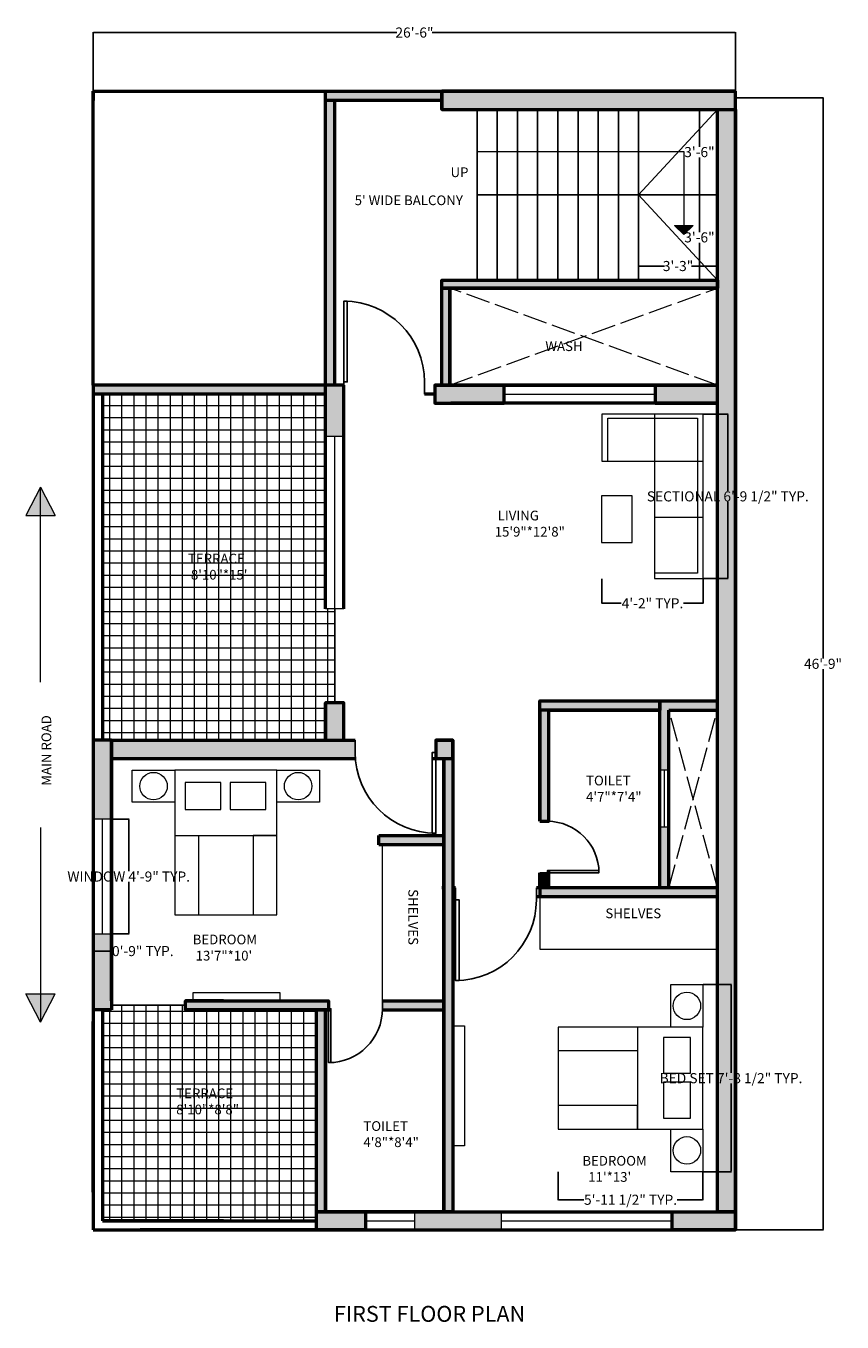
# Model space of a CAD drawing. Units: inches. Extents: x 292 to 1263, y 552 to 1204.
# Tile 3 of 3: x 859 to 1263, y 554 to 1196. Entities that reach past the tile are written whole.
import ezdxf

# ---------------------------------------------------------------- set-up
doc = ezdxf.new("R2010")
doc.units = ezdxf.units.IN
doc.header["$MEASUREMENT"] = 0
doc.linetypes.add('ACAD_ISO02W100', pattern=[15, 12, -3])
for name, color, linetype, lineweight in [('A-ANNO-DIMS', 2, 'Continuous', 18), ('A-ANNO-SYMB', 7, 'Continuous', 18), ('A-AREA-IDEN', 30, 'Continuous', 18), ('A-FLOR-CASE', 92, 'Continuous', 18), ('A-FLOR-OVHD', 8, 'ACAD_ISO02W100', 18), ('A-FLOR-PATT', 252, 'Continuous', 13), ('A-FLOR-STRS', 7, 'Continuous', 25), ('A-WALL-PATT', 22, 'Continuous', 13), ('DOOR', 200, 'Continuous', 25), ('FUR', 92, 'Continuous', 18), ('TEXT', 30, 'Continuous', 18), ('WALL', 22, 'Continuous', 50), ('WIND', 120, 'Continuous', 18)]:
    doc.layers.add(name, color=color, linetype=linetype, lineweight=lineweight)
doc.styles.get("Standard").update_dxf_attribs({"font": 'arial.ttf'})
doc.dimstyles.get("Standard").update_dxf_attribs({"dimtxt": 5, "dimasz": 0.18, "dimexe": 0.18, "dimexo": 0.0625, "dimgap": 0.09, "dimtad": 0, "dimtih": 1, "dimtoh": 1, "dimdec": 0, "dimzin": 0, "dimdsep": 46, "dimlunit": 4, "dimtxsty": 'Standard', "dimcen": 0.09, "dimadec": 0, "dimazin": 0, "dimtfac": 1, "dimtdec": 0, "dimtofl": 0, "dimtmove": 0, "dimatfit": 3, "dimfxl": 1, "dimtolj": 1, "dimtzin": 0, "dimarcsym": 0})

# ---------------------------------------------------------------- blocks, each defined once
blk = doc.blocks.new('*U2')
for p, q in [((0, 0), (0, -6)), ((40, 0), (40, -6))]:
    blk.add_line(p, q)
blk.add_lwpolyline([(0, 0), (0, 40), (1.75, 40), (1.75, 0)], close=True)
blk.add_arc((0, 0), 40, 0, 90)
blk = doc.blocks.new('*D8')
at = {"layer": 'A-ANNO-DIMS', "color": 0, "lineweight": -2, "transparency": 16777216}
for p, q in [((891.85, 1163.71), (891.85, 1192.9)), ((892.03, 1192.72), (1042.13, 1192.72)), ((1209.67, 1192.72), (1059.58, 1192.72)), ((1209.85, 1163.71), (1209.85, 1192.9))]:
    blk.add_line(p, q, dxfattribs=at)
at = {"layer": 'A-ANNO-DIMS', "color": 0, "lineweight": 100, "transparency": 16777216}
for points in [[(892.03, 1192.75), (892.03, 1192.69), (891.85, 1192.72)], [(1209.67, 1192.75), (1209.67, 1192.69), (1209.85, 1192.72)]]:
    blk.add_solid(points, dxfattribs=at)
at = {"layer": 'Defpoints', "color": 0, "lineweight": 100, "transparency": 16777216}
for p in [(1209.85, 1192.72), (891.85, 1163.64), (1209.85, 1163.64)]:
    blk.add_point(p, dxfattribs=at)
at = {"layer": 'A-ANNO-DIMS', "color": 0, "transparency": 16777216, "insert": (1050.85, 1192.72), "char_height": 5, "attachment_point": 5}
blk.add_mtext('\\A1;26\'-6"', dxfattribs=at)
blk = doc.blocks.new('*D9')
at = {"layer": 'A-ANNO-DIMS', "color": 0, "lineweight": -2, "transparency": 16777216}
for p, q in [((1209.92, 1160.44), (1253.31, 1160.44)), ((1253.13, 1160.26), (1253.13, 882.68)), ((1253.13, 599.82), (1253.13, 877.4)), ((1209.92, 599.64), (1253.31, 599.64))]:
    blk.add_line(p, q, dxfattribs=at)
at = {"layer": 'A-ANNO-DIMS', "color": 0, "lineweight": 100, "transparency": 16777216}
for points in [[(1253.1, 1160.26), (1253.16, 1160.26), (1253.13, 1160.44)], [(1253.1, 599.82), (1253.16, 599.82), (1253.13, 599.64)]]:
    blk.add_solid(points, dxfattribs=at)
at = {"layer": 'Defpoints', "color": 0, "lineweight": 100, "transparency": 16777216}
for p in [(1209.85, 1160.44), (1209.85, 599.64), (1253.13, 599.64)]:
    blk.add_point(p, dxfattribs=at)
at = {"layer": 'A-ANNO-DIMS', "color": 0, "transparency": 16777216, "insert": (1253.13, 880.04), "char_height": 5, "attachment_point": 5}
blk.add_mtext('\\A1;46\'-9"', dxfattribs=at)
blk = doc.blocks.new('*D10')
at = {"layer": 'A-ANNO-DIMS', "color": 0, "lineweight": -2, "transparency": 16777216}
for p, q in [((1200.79, 1112.39), (1191.75, 1112.39)), ((1191.93, 1112.21), (1191.93, 1093.91)), ((1191.93, 1070.32), (1191.93, 1088.62)), ((1200.79, 1070.14), (1191.75, 1070.14))]:
    blk.add_line(p, q, dxfattribs=at)
at = {"layer": 'A-ANNO-DIMS', "color": 0, "lineweight": 100, "transparency": 16777216}
for points in [[(1191.9, 1112.21), (1191.96, 1112.21), (1191.93, 1112.39)], [(1191.9, 1070.32), (1191.96, 1070.32), (1191.93, 1070.14)]]:
    blk.add_solid(points, dxfattribs=at)
at = {"layer": 'Defpoints', "color": 0, "lineweight": 100, "transparency": 16777216}
for p in [(1200.85, 1112.39), (1191.93, 1070.14), (1200.85, 1070.14)]:
    blk.add_point(p, dxfattribs=at)
at = {"layer": 'A-ANNO-DIMS', "color": 0, "transparency": 16777216, "insert": (1191.93, 1091.27), "char_height": 5, "attachment_point": 5}
blk.add_mtext('\\A1;3\'-6"', dxfattribs=at)
blk = doc.blocks.new('*D11')
at = {"layer": 'A-ANNO-DIMS', "color": 0, "lineweight": -2, "transparency": 16777216}
for p, q in [((1161.85, 1070.21), (1161.85, 1077.25)), ((1162.03, 1077.07), (1174.62, 1077.07)), ((1200.67, 1077.07), (1188.09, 1077.07)), ((1200.85, 1070.21), (1200.85, 1077.25))]:
    blk.add_line(p, q, dxfattribs=at)
at = {"layer": 'A-ANNO-DIMS', "color": 0, "lineweight": 100, "transparency": 16777216}
for points in [[(1162.03, 1077.1), (1162.03, 1077.04), (1161.85, 1077.07)], [(1200.67, 1077.1), (1200.67, 1077.04), (1200.85, 1077.07)]]:
    blk.add_solid(points, dxfattribs=at)
at = {"layer": 'Defpoints', "color": 0, "lineweight": 100, "transparency": 16777216}
for p in [(1200.85, 1077.07), (1161.85, 1070.14), (1200.85, 1070.14)]:
    blk.add_point(p, dxfattribs=at)
at = {"layer": 'A-ANNO-DIMS', "color": 0, "transparency": 16777216, "insert": (1181.35, 1077.07), "char_height": 5, "attachment_point": 5}
blk.add_mtext('\\A1;3\'-3"', dxfattribs=at)
blk = doc.blocks.new('*D12')
at = {"layer": 'A-ANNO-DIMS', "color": 0, "lineweight": -2, "transparency": 16777216}
for p, q in [((1200.79, 1154.64), (1191.75, 1154.64)), ((1191.93, 1154.46), (1191.93, 1136.16)), ((1191.93, 1112.57), (1191.93, 1130.87)), ((1200.79, 1112.39), (1191.75, 1112.39))]:
    blk.add_line(p, q, dxfattribs=at)
at = {"layer": 'A-ANNO-DIMS', "color": 0, "lineweight": 100, "transparency": 16777216}
for points in [[(1191.9, 1154.46), (1191.96, 1154.46), (1191.93, 1154.64)], [(1191.9, 1112.57), (1191.96, 1112.57), (1191.93, 1112.39)]]:
    blk.add_solid(points, dxfattribs=at)
at = {"layer": 'Defpoints', "color": 0, "lineweight": 100, "transparency": 16777216}
for p in [(1191.93, 1154.64), (1200.85, 1154.64), (1200.85, 1112.39)]:
    blk.add_point(p, dxfattribs=at)
at = {"layer": 'A-ANNO-DIMS', "color": 0, "transparency": 16777216, "insert": (1191.93, 1133.52), "char_height": 5, "attachment_point": 5}
blk.add_mtext('\\A1;3\'-6"', dxfattribs=at)
blk = doc.blocks.new('BED-DOUBLE')
for p, q in [((39.36, 71.59), (39.36, 21.08)), ((39.36, 71.59), (39.36, 59.89)), ((39.36, 59.89), (0, 59.89)), ((39.36, 32.73), (0, 32.73)), ((39.36, 21.08), (39.36, 32.73))]:
    blk.add_line(p, q)
for points in [[(71.7, 71.59), (55.84, 71.59), (55.84, 92.67), (71.7, 92.67)], [(71.7, 71.59), (0, 71.59), (0, 21.08), (71.7, 21.08)], [(65.61, 66.52), (52.22, 66.52), (52.22, 48.76), (65.61, 48.76)], [(65.61, 44.26), (52.22, 44.26), (52.22, 26.51), (65.61, 26.51)], [(71.7, 0), (55.84, 0), (55.84, 21.08), (71.7, 21.08)]]:
    blk.add_lwpolyline(points, close=True)
for centre in [(63.77, 82.13), (63.77, 10.54)]:
    blk.add_circle(centre, 6.81)
blk = doc.blocks.new('SOFA-SECTIONAL')
for p, q in [((2.73, 2.04), (2.73, 78.73)), ((2.73, 78.73), (24.15, 78.73)), ((24.15, 51.12), (0, 51.12)), ((47.26, 23.35), (47.26, 2.04)), ((47.26, 2.04), (2.73, 2.04))]:
    blk.add_line(p, q)
for points in [[(0, 0), (24.15, 0), (24.15, 81.48), (0, 81.48)], [(0, 0), (50.13, 0), (50.13, 23.35), (0, 23.35)]]:
    blk.add_lwpolyline(points, close=True)
blk = doc.blocks.new('STAIR-RETURN')
for p, q in [((0, 0), (0, 84.5)), ((10, 0), (10, 84.5)), ((20, 0), (20, 84.5)), ((30, 0), (30, 84.5)), ((40, 0), (40, 84.5)), ((50, 0), (50, 84.5)), ((60, 0), (60, 84.5)), ((70, 0), (70, 84.5)), ((80, 0), (80, 84.5)), ((80, 42.25), (119, 84.5)), ((0, 42.25), (119, 42.25)), ((80, 42.25), (119, 0)), ((80, 0), (80, 39))]:
    blk.add_line(p, q)
blk = doc.blocks.new('STAIR-TRAVEL-ARROW')
h = blk.add_hatch()
h.set_pattern_fill('ANSI31', color=256)
h.set_pattern_definition([(45, (-547.968, -1092.695), (-0.088388348, 0.088388348), [])])
h.paths.add_polyline_path([(102.33, 4.46), (97.71, 4.46), (102.33, 0)])
h.paths.add_polyline_path([(106.95, 4.46), (102.33, 4.46), (102.33, 0)])
for p, q in [((0, 41.14), (102.33, 41.14)), ((102.33, 41.14), (102.33, 0)), ((102.33, 0), (97.71, 4.46)), ((97.71, 4.46), (106.95, 4.46)), ((102.33, 0), (106.95, 4.46))]:
    blk.add_line(p, q)
blk = doc.blocks.new('ROAD-DIRECTION')
h = blk.add_hatch(color=256)
h.dxf.hatch_style = 1
h.paths.add_polyline_path([(7.26, 265.02), (0, 250.97), (7.26, 250.97)])
h.paths.add_polyline_path([(7.26, 265.02), (7.26, 250.97), (14.53, 250.97)])
h.paths.add_polyline_path([(14.53, 14.04), (7.26, 14.04), (7.26, 0)])
h.paths.add_polyline_path([(7.26, 14.04), (0, 14.04), (7.26, 0)])
for p, q in [((7.26, 265.02), (0, 250.97)), ((7.26, 168.49), (7.26, 265.02)), ((7.26, 265.02), (14.53, 250.97)), ((0, 250.97), (14.53, 250.97)), ((7.26, 96.52), (7.26, 0)), ((7.26, 0), (0, 14.04)), ((0, 14.04), (14.53, 14.04)), ((7.26, 0), (14.53, 14.04))]:
    blk.add_line(p, q)
blk = doc.blocks.new('WASH-VOID')
for p, q in [((0, 0), (132.5, 48)), ((132.5, 0), (0, 48))]:
    blk.add_line(p, q)
blk = doc.blocks.new('WIN-SIDE')
blk.add_line((4.5, 0), (4.5, 56.83))
blk.add_lwpolyline([(9, 56.83), (0, 56.83), (0, 0), (9, 0)], close=True)
blk = doc.blocks.new('WIN-BATH-NARROW')
blk.add_line((0, 4.5), (24.24, 4.5))
blk.add_lwpolyline([(0, 9), (24.24, 9), (24.24, 0), (0, 0)], close=True)
blk = doc.blocks.new('WIN-BEDROOM-WIDE')
blk.add_line((0, 4.5), (84.61, 4.5))
blk.add_lwpolyline([(0, 9), (84.61, 9), (84.61, 0), (0, 0)], close=True)
blk = doc.blocks.new('*D27')
at = {"layer": 'A-ANNO-DIMS', "color": 0, "lineweight": -2, "transparency": 16777216}
for p, q in [((1193.73, 721.15), (1207.75, 721.15)), ((1207.57, 720.97), (1207.57, 677.49)), ((1207.57, 628.66), (1207.57, 672.14)), ((1193.73, 628.48), (1207.75, 628.48))]:
    blk.add_line(p, q, dxfattribs=at)
at = {"layer": 'A-ANNO-DIMS', "color": 0, "lineweight": 100, "transparency": 16777216}
for points in [[(1207.54, 720.97), (1207.6, 720.97), (1207.57, 721.15)], [(1207.54, 628.66), (1207.6, 628.66), (1207.57, 628.48)]]:
    blk.add_solid(points, dxfattribs=at)
at = {"layer": 'Defpoints', "color": 0, "lineweight": 100, "transparency": 16777216}
for p in [(1193.67, 721.15), (1207.57, 721.15), (1193.67, 628.48)]:
    blk.add_point(p, dxfattribs=at)
at = {"layer": 'A-ANNO-DIMS', "color": 0, "transparency": 16777216, "insert": (1207.57, 674.81), "char_height": 5, "attachment_point": 5}
blk.add_mtext('\\A1;BED SET 7\'-8 1/2" TYP.', dxfattribs=at)
blk = doc.blocks.new('*D28')
at = {"layer": 'A-ANNO-DIMS', "color": 0, "lineweight": -2, "transparency": 16777216}
for p, q in [((1121.97, 628.41), (1121.97, 614.4)), ((1193.67, 628.41), (1193.67, 614.4)), ((1122.15, 614.58), (1134.73, 614.58)), ((1193.49, 614.58), (1180.92, 614.58))]:
    blk.add_line(p, q, dxfattribs=at)
at = {"layer": 'A-ANNO-DIMS', "color": 0, "lineweight": 100, "transparency": 16777216}
for points in [[(1122.15, 614.61), (1122.15, 614.55), (1121.97, 614.58)], [(1193.49, 614.61), (1193.49, 614.55), (1193.67, 614.58)]]:
    blk.add_solid(points, dxfattribs=at)
at = {"layer": 'Defpoints', "color": 0, "lineweight": 100, "transparency": 16777216}
for p in [(1121.97, 628.48), (1193.67, 628.48), (1193.67, 614.58)]:
    blk.add_point(p, dxfattribs=at)
at = {"layer": 'A-ANNO-DIMS', "color": 0, "transparency": 16777216, "insert": (1157.82, 614.58), "char_height": 5, "attachment_point": 5}
blk.add_mtext('\\A1;5\'-11 1/2" TYP.', dxfattribs=at)
blk = doc.blocks.new('*D33')
at = {"layer": 'A-ANNO-DIMS', "color": 0, "lineweight": -2, "transparency": 16777216}
for p, q in [((900.92, 803.1), (909.56, 803.1)), ((909.38, 802.92), (909.38, 777.36)), ((909.38, 746.45), (909.38, 772.01)), ((900.92, 746.27), (909.56, 746.27))]:
    blk.add_line(p, q, dxfattribs=at)
at = {"layer": 'A-ANNO-DIMS', "color": 0, "lineweight": 100, "transparency": 16777216}
for points in [[(909.35, 802.92), (909.41, 802.92), (909.38, 803.1)], [(909.35, 746.45), (909.41, 746.45), (909.38, 746.27)]]:
    blk.add_solid(points, dxfattribs=at)
at = {"layer": 'Defpoints', "color": 0, "lineweight": 100, "transparency": 16777216}
for p in [(900.85, 803.1), (909.38, 803.1), (900.85, 746.27)]:
    blk.add_point(p, dxfattribs=at)
at = {"layer": 'A-ANNO-DIMS', "color": 0, "transparency": 16777216, "insert": (909.38, 774.68), "char_height": 5, "attachment_point": 5}
blk.add_mtext('\\A1;WINDOW 4\'-9" TYP.', dxfattribs=at)
blk = doc.blocks.new('*D34')
at = {"layer": 'A-ANNO-DIMS', "color": 0, "lineweight": -2, "transparency": 16777216}
for p, q in [((891.85, 746.21), (891.85, 737.57)), ((900.85, 746.21), (900.85, 737.57)), ((892.03, 737.75), (900.67, 737.75)), ((900.85, 737.75), (901.03, 737.75))]:
    blk.add_line(p, q, dxfattribs=at)
at = {"layer": 'A-ANNO-DIMS', "color": 0, "lineweight": 100, "transparency": 16777216}
for points in [[(892.03, 737.78), (892.03, 737.72), (891.85, 737.75)], [(900.67, 737.78), (900.67, 737.72), (900.85, 737.75)]]:
    blk.add_solid(points, dxfattribs=at)
at = {"layer": 'Defpoints', "color": 0, "lineweight": 100, "transparency": 16777216}
for p in [(891.85, 746.27), (900.85, 746.27), (900.85, 737.75)]:
    blk.add_point(p, dxfattribs=at)
at = {"layer": 'A-ANNO-DIMS', "color": 0, "transparency": 16777216, "insert": (916.36, 737.75), "char_height": 5, "attachment_point": 5}
blk.add_mtext('\\A1;0\'-9" TYP.', dxfattribs=at)
blk = doc.blocks.new('*D35')
at = {"layer": 'A-ANNO-DIMS', "color": 0, "lineweight": -2, "transparency": 16777216}
for p, q in [((1193.83, 1003.72), (1206.17, 1003.72)), ((1205.99, 1003.54), (1205.99, 965.66)), ((1205.99, 922.42), (1205.99, 960.3)), ((1193.83, 922.24), (1206.17, 922.24))]:
    blk.add_line(p, q, dxfattribs=at)
at = {"layer": 'A-ANNO-DIMS', "color": 0, "lineweight": 100, "transparency": 16777216}
for points in [[(1205.96, 1003.54), (1206.02, 1003.54), (1205.99, 1003.72)], [(1205.96, 922.42), (1206.02, 922.42), (1205.99, 922.24)]]:
    blk.add_solid(points, dxfattribs=at)
at = {"layer": 'Defpoints', "color": 0, "lineweight": 100, "transparency": 16777216}
for p in [(1193.77, 1003.72), (1193.77, 922.24), (1205.99, 922.24)]:
    blk.add_point(p, dxfattribs=at)
at = {"layer": 'A-ANNO-DIMS', "color": 0, "transparency": 16777216, "insert": (1205.99, 962.98), "char_height": 5, "attachment_point": 5}
blk.add_mtext('\\A1;SECTIONAL 6\'-9 1/2" TYP.', dxfattribs=at)
blk = doc.blocks.new('*D36')
at = {"layer": 'A-ANNO-DIMS', "color": 0, "lineweight": -2, "transparency": 16777216}
for p, q in [((1143.64, 922.18), (1143.64, 909.84)), ((1193.77, 922.18), (1193.77, 909.84)), ((1143.82, 910.02), (1153.27, 910.02)), ((1193.59, 910.02), (1184.13, 910.02))]:
    blk.add_line(p, q, dxfattribs=at)
at = {"layer": 'A-ANNO-DIMS', "color": 0, "lineweight": 100, "transparency": 16777216}
for points in [[(1143.82, 910.05), (1143.82, 909.99), (1143.64, 910.02)], [(1193.59, 910.05), (1193.59, 909.99), (1193.77, 910.02)]]:
    blk.add_solid(points, dxfattribs=at)
at = {"layer": 'Defpoints', "color": 0, "lineweight": 100, "transparency": 16777216}
for p in [(1143.64, 922.24), (1193.77, 922.24), (1143.64, 910.02)]:
    blk.add_point(p, dxfattribs=at)
at = {"layer": 'A-ANNO-DIMS', "color": 0, "transparency": 16777216, "insert": (1168.7, 910.02), "char_height": 5, "attachment_point": 5}
blk.add_mtext('\\A1;4\'-2" TYP.', dxfattribs=at)

msp = doc.modelspace()

# ---------------------------------------------------------------- hatches: boundary and pattern name
at = {"layer": 'A-FLOR-PATT'}
h = msp.add_hatch(dxfattribs=at)
h.set_pattern_fill('NET', color=256, scale=48)
h.paths.add_polyline_path([(1006.85, 992.78), (1006.85, 1013.64), (896.35, 1013.64), (896.35, 842.14), (900.85, 842.14), (1006.85, 842.14), (1006.85, 860.7), (1011.35, 860.7), (1011.35, 907.34), (1006.85, 907.34)])
h = msp.add_hatch(dxfattribs=at)
h.set_pattern_fill('NET', color=256, scale=48)
h.paths.add_polyline_path([(1002.35, 708.64), (960.85, 708.64), (937.46, 708.64), (937.46, 710.89), (900.85, 710.89), (900.85, 708.64), (896.35, 708.64), (896.35, 604.14), (1002.35, 604.14)])
at = {"layer": 'A-WALL-PATT'}
h = msp.add_hatch(color=256, dxfattribs=at)
h.dxf.hatch_style = 1
h.paths.add_polyline_path([(1064.35, 1163.64), (1006.85, 1163.64), (1006.85, 1159.14), (1064.35, 1159.14)])
h.paths.add_polyline_path([(1011.35, 1159.14), (1006.85, 1159.14), (1006.85, 1018.14), (1011.35, 1018.14)])
h.paths.add_polyline_path([(1015.85, 1018.14), (1006.85, 1018.14), (1006.85, 992.78), (1015.85, 992.78)])
h.paths.add_polyline_path([(1015.85, 860.7), (1006.85, 860.7), (1006.85, 842.14), (1015.85, 842.14)])
h.paths.add_polyline_path([(1021.45, 842.14), (900.85, 842.14), (900.85, 833.14), (1021.56, 833.14, -0.01877), (1021.45, 836.14)])
h.paths.add_polyline_path([(900.85, 833.14), (900.85, 842.14), (891.85, 842.14), (891.85, 803.1), (900.85, 803.1)])
h.paths.add_polyline_path([(900.85, 746.27), (891.85, 746.27), (891.85, 708.64), (900.85, 708.64), (900.85, 713.14)])
h.paths.add_polyline_path([(1093.9, 608.64), (1050.85, 608.64), (1050.85, 599.64), (1093.9, 599.64)])
h.paths.add_polyline_path([(1065.35, 713.14), (1034.99, 713.14), (1034.99, 709.15, -0.004712), (1034.99, 708.64), (1065.35, 708.64)])
h.paths.add_polyline_path([(1065.35, 794.94), (1033.18, 794.94), (1033.18, 790.44), (1065.35, 790.44)])
h.paths.add_polyline_path([(1200.85, 769.14), (1176.85, 769.14), (1117.35, 769.14), (1112.85, 769.14), (1112.85, 764.64), (1200.85, 764.64)])
h.paths.add_polyline_path([(1176.85, 857.14), (1200.85, 857.14), (1200.85, 861.64), (1172.35, 861.64), (1172.35, 827.48), (1176.85, 827.48)])
h.paths.add_polyline_path([(1176.85, 799.1), (1172.35, 799.1), (1172.35, 769.14), (1176.85, 769.14)])
h = msp.add_hatch(color=256, dxfattribs=at)
h.dxf.hatch_style = 1
h.paths.add_polyline_path([(1200.85, 1070.14), (1064.35, 1070.14), (1064.35, 1066.14), (1068.35, 1066.14), (1200.85, 1066.14)])
h.paths.add_polyline_path([(1068.35, 1066.14), (1064.35, 1066.14), (1064.35, 1018.14), (1068.35, 1018.14)])
h.paths.add_polyline_path([(1095.23, 1018.14), (1060.89, 1018.14), (1060.89, 1009.14), (1095.23, 1009.14)])
h.paths.add_polyline_path([(1200.85, 1018.14), (1170.03, 1018.14), (1170.03, 1009.14), (1200.85, 1009.14)])
h.paths.add_polyline_path([(1209.85, 1154.64), (1200.85, 1154.64), (1200.85, 608.64), (1209.85, 608.64)])
h.paths.add_polyline_path([(1209.85, 1163.64), (1064.35, 1163.64), (1064.35, 1154.64), (1209.85, 1154.64)])
h.paths.add_polyline_path([(1117.35, 857.14), (1112.85, 857.14), (1112.85, 802.03), (1117.35, 802.03)])
h.paths.add_polyline_path([(1172.35, 861.64), (1112.85, 861.64), (1112.85, 857.14), (1117.35, 857.14), (1172.35, 857.14)])
h.paths.add_polyline_path([(1069.85, 842.14), (1061.45, 842.14), (1061.45, 833.14), (1069.85, 833.14)])
h.paths.add_polyline_path([(1069.85, 833.14), (1065.35, 833.14), (1065.35, 608.64), (1069.85, 608.64)])
h.paths.add_polyline_path([(1008.34, 713.14), (937.46, 713.14), (937.46, 708.64), (1008.34, 708.64)])
h.paths.add_polyline_path([(1006.85, 708.64), (1002.35, 708.64), (1002.35, 608.64), (1006.85, 608.64)])
h.paths.add_polyline_path([(1026.62, 608.64), (1002.35, 608.64), (1002.35, 599.64), (1026.62, 599.64)])
h.paths.add_polyline_path([(1209.85, 608.64), (1200.85, 608.64), (1178.51, 608.64), (1178.51, 599.64), (1209.85, 599.64)])
h = msp.add_hatch(color=256, dxfattribs=at)
h.dxf.hatch_style = 1
h.paths.add_polyline_path([(1006.85, 1018.14), (891.85, 1018.14), (891.85, 1013.64), (1006.85, 1013.64)])
h = msp.add_hatch(color=256, dxfattribs=at)
h.dxf.hatch_style = 1
h.paths.add_polyline_path([(1117.35, 776.52), (1116.68, 776.52), (1112.85, 776.52), (1112.85, 769.14), (1117.35, 769.14)])

# ---------------------------------------------------------------- linework, layer by layer
at = {"layer": 'A-FLOR-CASE'}
for p, q in [((1034.99, 713.14), (1034.99, 790.44)), ((1112.85, 764.64), (1112.85, 738.68)), ((1112.85, 738.68), (1200.85, 738.68))]:
    msp.add_line(p, q, dxfattribs=at)
at = {"layer": 'A-FLOR-OVHD'}
for p, q in [((1176.85, 769.14), (1200.85, 857.14)), ((1200.85, 769.14), (1176.85, 857.14))]:
    msp.add_line(p, q, dxfattribs=at)
at = {"layer": 'A-FLOR-STRS'}
msp.add_line((1200.85, 1070.14), (1161.85, 1070.14), dxfattribs=at)
msp.add_line((1200.85, 1070.14), (1161.85, 1070.14), dxfattribs=at)
at = {"layer": 'DOOR'}
for p, q in [((1011.35, 860.7), (1011.35, 907.34)), ((937.46, 710.89), (900.85, 710.89))]:
    msp.add_line(p, q, dxfattribs=at)
at = {"layer": 'FUR'}
for points in [[(1158.62, 963.19), (1143.44, 963.19), (1143.44, 940.09), (1158.62, 940.09)], [(941.17, 713.14), (984.32, 713.14), (984.32, 717.07), (941.17, 717.07)], [(1069.85, 700.76), (1075.56, 700.76), (1075.56, 641.23), (1069.85, 641.23)]]:
    msp.add_lwpolyline(points, close=True, dxfattribs=at)
at = {"layer": 'WALL'}
for p, q in [((891.85, 1163.64), (1209.85, 1163.64)), ((891.85, 1163.64), (891.85, 1159.14)), ((891.85, 1018.14), (891.85, 1163.64)), ((1006.85, 1159.14), (1006.85, 1163.64)), ((1064.35, 1154.64), (1064.35, 1163.64)), ((1209.85, 599.64), (1209.85, 1163.64)), ((1064.35, 1159.14), (1006.85, 1159.14)), ((1006.85, 1018.14), (1006.85, 1159.14)), ((1011.35, 1018.14), (1011.35, 1159.14)), ((1064.35, 1154.64), (1200.85, 1154.64)), ((1200.85, 608.64), (1200.85, 1154.64)), ((1064.35, 1018.14), (1064.35, 1070.14)), ((1064.35, 1070.14), (1200.85, 1070.14)), ((1068.35, 1018.14), (1068.35, 1066.14)), ((1068.35, 1066.14), (1200.85, 1066.14)), ((891.85, 1018.14), (891.85, 1038.14)), ((891.85, 1018.14), (891.85, 599.64)), ((1006.85, 1018.14), (891.85, 1018.14)), ((1015.85, 1018.14), (1006.85, 1018.14)), ((1006.85, 907.34), (1006.85, 1018.14)), ((1015.85, 907.34), (1015.85, 1018.14)), ((1060.89, 1018.14), (1068.35, 1018.14)), ((1060.89, 1018.14), (1060.89, 1009.14)), ((1063.85, 1018.14), (1200.85, 1018.14)), ((1200.85, 1018.14), (1068.85, 1018.14)), ((1006.85, 1013.64), (891.85, 1013.64)), ((1060.89, 1013.64), (1055.85, 1013.64)), ((1060.89, 1009.14), (1071.97, 1009.14)), ((1200.85, 1009.14), (1068.85, 1009.14)), ((1006.85, 842.14), (1006.85, 860.7)), ((1015.85, 842.14), (1015.85, 860.7)), ((1112.85, 861.64), (1172.35, 861.64)), ((1112.85, 802.03), (1112.85, 861.64)), ((1172.35, 769.14), (1172.35, 861.64)), ((1172.35, 861.64), (1200.85, 861.64)), ((1117.35, 857.14), (1172.35, 857.14)), ((1117.35, 802.02), (1117.35, 857.14)), ((1176.85, 769.14), (1176.85, 857.14)), ((1176.85, 857.14), (1200.85, 857.14)), ((900.85, 842.14), (891.85, 842.14)), ((900.85, 837.64), (900.85, 842.14)), ((900.85, 713.14), (900.85, 842.14)), ((900.85, 842.14), (1021.45, 842.14)), ((900.85, 842.14), (1006.85, 842.14)), ((900.85, 842.14), (900.85, 708.64)), ((1061.45, 842.14), (1065.35, 842.14)), ((1065.35, 842.14), (1069.85, 842.14)), ((1069.85, 842.14), (1069.85, 608.64)), ((900.85, 713.14), (900.85, 833.14)), ((900.85, 713.14), (900.85, 833.14)), ((900.85, 833.14), (1021.56, 833.14)), ((1059.7, 833.14), (1065.35, 833.14)), ((1065.35, 833.14), (1065.35, 608.64)), ((1033.18, 790.44), (1033.18, 794.94)), ((1033.18, 794.94), (1065.35, 794.94)), ((1065.35, 790.44), (1033.18, 790.44)), ((1117.35, 769.14), (1117.35, 777.64)), ((1112.85, 769.14), (1112.85, 776.52)), ((1065.35, 769.14), (1064.35, 769.14)), ((1071.23, 769.14), (1069.85, 769.14)), ((1071.23, 764.64), (1069.85, 764.64)), ((1117.35, 769.14), (1111.23, 769.14)), ((1112.85, 764.64), (1111.23, 764.64)), ((1112.85, 769.14), (1112.85, 764.64)), ((1200.85, 764.64), (1112.85, 764.64)), ((1200.85, 769.14), (1117.35, 769.14)), ((1172.35, 769.14), (1117.35, 769.14)), ((1200.85, 769.14), (1176.85, 769.14)), ((1200.85, 608.64), (1200.85, 764.64)), ((1200.85, 608.64), (1200.85, 764.64)), ((1200.85, 608.64), (1200.85, 737.64)), ((956.35, 713.14), (937.46, 713.14)), ((937.46, 713.14), (1008.34, 713.14)), ((956.35, 713.14), (1008.34, 713.14)), ((1034.99, 713.14), (1065.35, 713.14)), ((1034.99, 713.14), (1063.85, 713.14)), ((900.85, 708.64), (891.85, 708.64)), ((896.35, 708.64), (896.35, 604.14)), ((960.85, 708.64), (937.46, 708.64)), ((960.85, 708.64), (1009.51, 708.64)), ((1002.35, 604.14), (1002.35, 708.64)), ((1006.85, 608.64), (1006.85, 708.64)), ((1034.99, 708.64), (1065.35, 708.64)), ((956.35, 604.14), (896.35, 604.14)), ((896.35, 604.14), (1002.35, 604.14)), ((1003.85, 608.64), (1002.35, 608.64)), ((1016.85, 608.64), (1002.35, 608.64)), ((1002.35, 608.64), (1200.85, 608.64)), ((1064.35, 608.64), (1008.35, 608.64)), ((891.85, 599.64), (1209.85, 599.64))]:
    msp.add_line(p, q, dxfattribs=at)
for points in [[(1209.85, 1163.64), (1064.35, 1163.64), (1064.35, 1154.64), (1209.85, 1154.64)], [(1209.85, 608.64), (1200.85, 608.64), (1200.85, 1154.64), (1209.85, 1154.64)], [(1200.85, 1066.14), (1064.35, 1066.14), (1064.35, 1070.14), (1200.85, 1070.14)], [(1064.35, 1066.14), (1068.35, 1066.14), (1068.35, 1018.14), (1064.35, 1018.14)], [(1095.23, 1018.14), (1060.89, 1018.14), (1060.89, 1009.14), (1095.23, 1009.14)], [(1170.03, 1009.14), (1200.85, 1009.14), (1200.85, 1018.14), (1170.03, 1018.14)], [(1006.85, 842.14), (1015.85, 842.14), (1015.85, 860.7), (1006.85, 860.7)], [(1172.35, 857.14), (1112.85, 857.14), (1112.85, 861.64), (1172.35, 861.64)], [(1112.85, 802.03), (1117.35, 802.03), (1117.35, 857.14), (1112.85, 857.14)], [(1061.45, 833.14), (1069.85, 833.14), (1069.85, 842.14), (1061.45, 842.14)], [(1065.35, 833.14), (1069.85, 833.14), (1069.85, 608.64), (1065.35, 608.64)], [(1008.34, 708.64), (937.46, 708.64), (937.46, 713.14), (1008.34, 713.14)], [(1006.85, 608.64), (1002.35, 608.64), (1002.35, 708.64), (1006.85, 708.64)], [(1026.62, 599.64), (1002.35, 599.64), (1002.35, 608.64), (1026.62, 608.64)], [(1178.51, 608.64), (1209.85, 608.64), (1209.85, 599.64), (1178.51, 599.64)]]:
    msp.add_lwpolyline(points, close=True, dxfattribs=at)
for points in [[(891.85, 1013.64), (891.85, 842.14)], [(896.35, 1013.64), (896.35, 842.14)], [(900.85, 713.14), (900.85, 708.64)], [(937.46, 708.64), (937.46, 713.14)], [(891.85, 618.29), (891.85, 702.82)], [(1002.35, 608.64), (1003.49, 608.64)], [(1003.49, 599.64), (915.01, 599.64)]]:
    msp.add_lwpolyline(points, dxfattribs=at)
at = {"layer": 'WIND'}
for p, q in [((1095.23, 1013.64), (1170.03, 1013.64)), ((1011.35, 907.34), (1011.35, 992.78)), ((1174.6, 799.1), (1174.6, 827.48))]:
    msp.add_line(p, q, dxfattribs=at)
for points in [[(1095.23, 1018.14), (1170.03, 1018.14), (1170.03, 1009.14), (1095.23, 1009.14)], [(1006.85, 992.78), (1015.85, 992.78), (1015.85, 907.34), (1006.85, 907.34)], [(1172.35, 827.48), (1176.85, 827.48), (1176.85, 799.1), (1172.35, 799.1)]]:
    msp.add_lwpolyline(points, close=True, dxfattribs=at)

# ---------------------------------------------------------------- block references
at = {"layer": 'A-ANNO-SYMB'}
for name, p in [('STAIR-TRAVEL-ARROW', (1081.85, 1092.69)), ('ROAD-DIRECTION', (858.5, 702.52))]:
    msp.add_blockref(name, p, dxfattribs=at)
at = {"layer": 'A-FLOR-OVHD'}
msp.add_blockref('WASH-VOID', (1068.35, 1018.14), dxfattribs=at)
at = {"layer": 'A-FLOR-STRS'}
msp.add_blockref('STAIR-RETURN', (1081.85, 1070.14), dxfattribs=at)
at = {"layer": 'DOOR'}
msp.add_blockref('*U2', (1015.85, 1019.64), dxfattribs=at)
at = {"layer": 'DOOR', "rotation": 180}
msp.add_blockref('*U2', (1061.45, 836.14), dxfattribs=at)
at = {"layer": 'DOOR'}
for p, xscale, yscale, zscale, rotation in [((1116.68, 776.52), -0.6376819810629283, 0.6376819810629283, 0.6376819810629283, 270), ((1008.34, 709.15), -0.6662897282403346, 0.6662897282403346, 0.6662897282403346, 180)]:
    msp.add_blockref('*U2', p, dxfattribs=dict(at, xscale=xscale, yscale=yscale, zscale=zscale, rotation=rotation))
at = {"layer": 'DOOR', "xscale": -1, "rotation": 180}
msp.add_blockref('*U2', (1071.23, 763.14), dxfattribs=at)
at = {"layer": 'FUR'}
for name, p, rotation in [('SOFA-SECTIONAL', (1193.77, 1003.72), 180), ('BED-DOUBLE', (1003.8, 755.69), 89.99999999999955)]:
    msp.add_blockref(name, p, dxfattribs=dict(at, rotation=rotation))
msp.add_blockref('BED-DOUBLE', (1121.97, 628.48), dxfattribs=at)
at = {"layer": 'WIND'}
for name, p in [('WIN-SIDE', (891.85, 746.27)), ('WIN-BATH-NARROW', (1026.62, 599.64)), ('WIN-BEDROOM-WIDE', (1093.9, 599.64))]:
    msp.add_blockref(name, p, dxfattribs=at)

# ---------------------------------------------------------------- texts
at = {"layer": 'A-AREA-IDEN', "attachment_point": 1}
for s, insert, char_height in [("5' WIDE BALCONY", (1021.25, 1112.03), 4.8055), ('WASH', (1115.67, 1039.76), 4.805), (' LIVING\\P15\'9"*12\'8"', (1090.58, 955.88), 4.8055), ('TERRACE\\P 8\'10"*15\'', (938.7, 934.57), 4.805), ('TOILET\\P4\'7"*7\'4"', (1135.81, 824.62), 4.805), ('BEDROOM\\P 13\'7"*10\'', (941.05, 745.9), 4.805), ('TERRACE\\P8\'10"*8\'8"', (932.91, 669.7), 4.805), ('TOILET\\P4\'8"*8\'4"', (1025.57, 653.49), 4.805), ("BEDROOM\\P  11'*13'", (1133.97, 636.28), 4.805)]:
    msp.add_mtext_dynamic_manual_height_columns(s, width=2330.1292, gutter_width=24.03, heights=[0], dxfattribs=dict(at, insert=insert, char_height=char_height))
at = {"layer": 'TEXT', "attachment_point": 1}
for s, width, gutter_width, insert, char_height in [('UP', 2330.1292, 24.03, (1068.72, 1125.92), 4.805), ('SHELVES', 2330.1292, 24.03, (1145.36, 758.85), 4.805), ('FIRST FLOOR PLAN', 3807.3933, 39.26, (1010.95, 561.98), 7.8521)]:
    msp.add_mtext_dynamic_manual_height_columns(s, width=width, gutter_width=gutter_width, heights=[0], dxfattribs=dict(at, insert=insert, char_height=char_height))
at = {"layer": 'TEXT', "char_height": 4.805, "attachment_point": 1}
for s, insert, rotation in [('MAIN ROAD', (866.21, 819.63), 90), ('SHELVES', (1052.65, 768.42), 270)]:
    msp.add_mtext_dynamic_manual_height_columns(s, width=2330.1292, gutter_width=24.03, heights=[0], dxfattribs=dict(at, insert=insert, rotation=rotation))

# ---------------------------------------------------------------- dimensions: what is measured, and where the dimension line sits
at = {"layer": 'A-ANNO-DIMS'}
for base, p1, p2, picture, middle in [((1209.85, 1192.72), (891.85, 1163.64), (1209.85, 1163.64), '*D8', (1050.85, 1192.72)), ((1200.85, 1077.07), (1161.85, 1070.14), (1200.85, 1070.14), '*D11', (1181.35, 1077.07))]:
    dim = msp.add_linear_dim(base=base, p1=p1, p2=p2, dimstyle='Standard', override={"dimclrd": 0, "dimclre": 0, "dimclrt": 0}, dxfattribs=at)
    dim.commit()
    dim.dimension.update_dxf_attribs({"geometry": picture, "text_midpoint": middle})
for base, p1, p2, picture, middle in [((1253.13, 599.64), (1209.85, 1160.44), (1209.85, 599.64), '*D9', (1253.13, 880.04)), ((1191.93, 1154.64), (1200.85, 1112.39), (1200.85, 1154.64), '*D12', (1191.93, 1133.52)), ((1191.93, 1070.14), (1200.85, 1112.39), (1200.85, 1070.14), '*D10', (1191.93, 1091.27))]:
    dim = msp.add_linear_dim(base=base, p1=p1, p2=p2, angle=90, dimstyle='Standard', override={"dimclrd": 0, "dimclre": 0, "dimclrt": 0}, dxfattribs=at)
    dim.commit()
    dim.dimension.update_dxf_attribs({"geometry": picture, "text_midpoint": middle})
for base, p1, p2, angle, text, picture, middle in [((1205.99, 922.24), (1193.77, 1003.72), (1193.77, 922.24), 270, 'SECTIONAL <> TYP.', '*D35', (1205.99, 962.98)), ((1143.64, 910.02), (1193.77, 922.24), (1143.64, 922.24), 180, '<> TYP.', '*D36', (1168.7, 910.02)), ((909.38, 803.1), (900.85, 746.27), (900.85, 803.1), 90, 'WINDOW <> TYP.', '*D33', (909.38, 774.68)), ((1207.57, 721.15), (1193.67, 628.48), (1193.67, 721.15), 90, 'BED SET <> TYP.', '*D27', (1207.57, 674.81))]:
    dim = msp.add_linear_dim(base=base, p1=p1, p2=p2, angle=angle, text=text, dimstyle='Standard', override={"dimdec": 1, "dimlfac": 1, "dimrnd": 0, "dimzin": 1, "dimdsep": 46, "dimlunit": 4, "dimfrac": 2}, dxfattribs=at)
    dim.commit()
    dim.dimension.update_dxf_attribs({"geometry": picture, "text_midpoint": middle})
for base, p1, p2, picture, middle in [((900.85, 737.75), (891.85, 746.27), (900.85, 746.27), '*D34', (916.36, 737.75)), ((1193.67, 614.58), (1121.97, 628.48), (1193.67, 628.48), '*D28', (1157.82, 614.58))]:
    dim = msp.add_linear_dim(base=base, p1=p1, p2=p2, text='<> TYP.', dimstyle='Standard', override={"dimdec": 1, "dimlfac": 1, "dimrnd": 0, "dimzin": 1, "dimdsep": 46, "dimlunit": 4, "dimfrac": 2}, dxfattribs=at)
    dim.commit()
    dim.dimension.update_dxf_attribs({"geometry": picture, "text_midpoint": middle})

doc.saveas('drawing.dxf')
